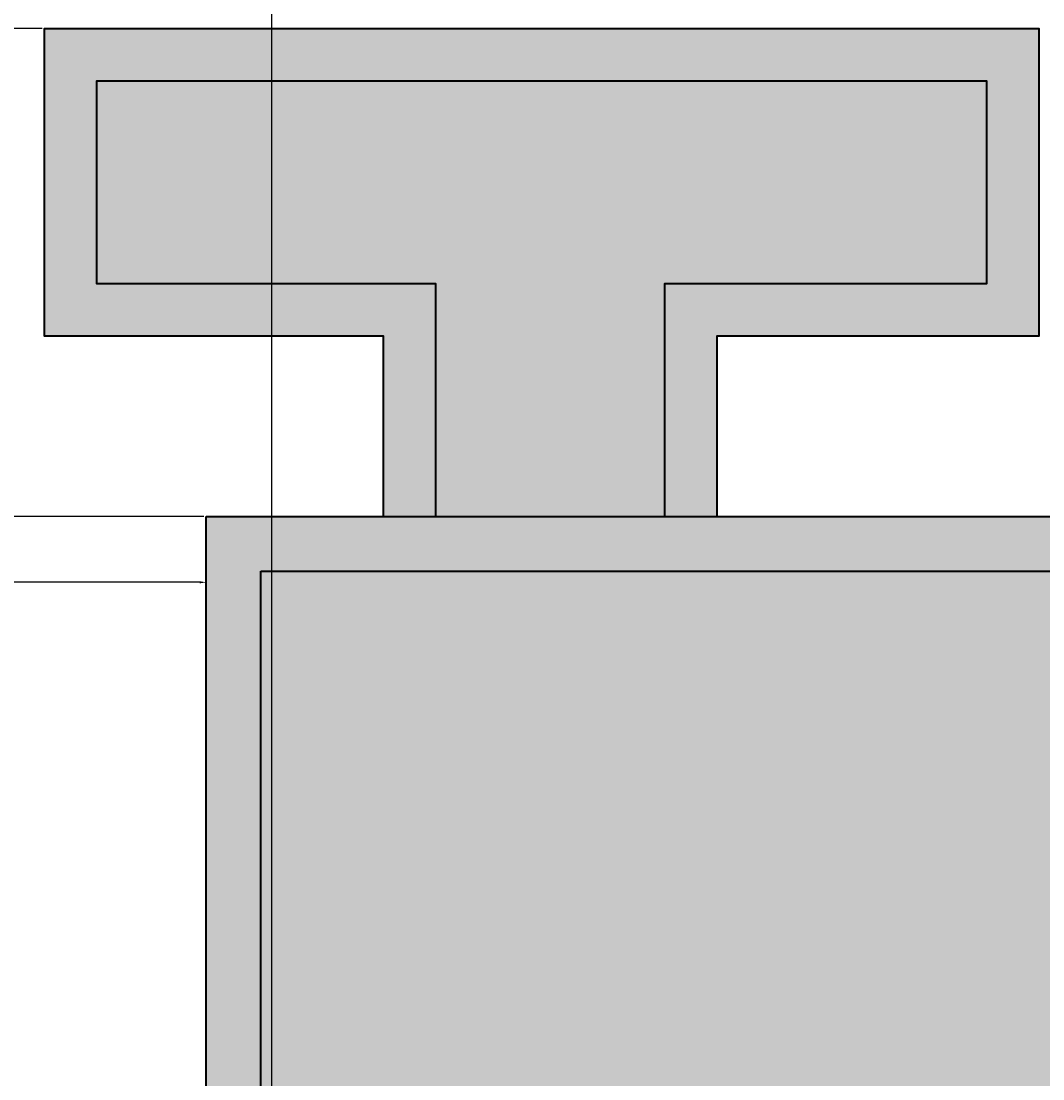
# Model space of a CAD drawing. Units: millimetres. Extents: x -11 to 280, y -4 to 208.
# Tile 15 of 55: x 24 to 52, y 164 to 193. Entities that reach past the tile are written whole.
import ezdxf

# ---------------------------------------------------------------- set-up
doc = ezdxf.new("R2010")
doc.units = ezdxf.units.MM
for name, color, linetype, lineweight in [('M-DIMS', 2, 'Continuous', 18), ('M-HYDR-EQPM', 7, 'Continuous', 35), ('M-HYDR-EQPM-PATT', 252, 'Continuous', 13)]:
    doc.layers.add(name, color=color, linetype=linetype, lineweight=lineweight)
doc.styles.get("Standard").update_dxf_attribs({"font": 'arial.ttf'})
doc.dimstyles.get("Standard").update_dxf_attribs({"dimtxt": 0.18, "dimasz": 0.18, "dimexe": 0.18, "dimexo": 0.0625, "dimgap": 0.09, "dimtad": 0, "dimtih": 1, "dimtoh": 1, "dimdec": 4, "dimzin": 0, "dimdsep": 46, "dimtxsty": 'Standard', "dimcen": 0.09, "dimadec": 0, "dimazin": 0, "dimtfac": 1, "dimtdec": 4, "dimtofl": 0, "dimtmove": 0, "dimatfit": 3, "dimfxl": 1, "dimtolj": 1, "dimtzin": 0, "dimarcsym": 0})

# ---------------------------------------------------------------- blocks, each defined once
blk = doc.blocks.new('*D5')
at = {"layer": 'Defpoints', "color": 0, "transparency": 16777216}
for p in [(24.759, 192.645), (-10.087, 11.435), (261.686, 11.435)]:
    blk.add_point(p, dxfattribs=at)
at = {"layer": 'M-DIMS', "color": 0, "lineweight": -2, "transparency": 16777216}
for p, q in [((24.696, 192.645), (-10.267, 192.645)), ((-10.087, 192.465), (-10.087, 102.222)), ((-10.087, 11.615), (-10.087, 101.858)), ((261.624, 11.435), (-10.267, 11.435))]:
    blk.add_line(p, q, dxfattribs=at)
at = {"layer": 'M-DIMS', "color": 0, "transparency": 16777216}
for points in [[(-10.117, 192.465), (-10.057, 192.465), (-10.087, 192.645)], [(-10.117, 11.615), (-10.057, 11.615), (-10.087, 11.435)]]:
    blk.add_solid(points, dxfattribs=at)
at = {"layer": 'M-DIMS', "color": 0, "transparency": 16777216, "insert": (-10.087, 102.04), "char_height": 0.18, "attachment_point": 5}
blk.add_mtext('\\A1;181.2', dxfattribs=at)
blk = doc.blocks.new('*D8')
at = {"layer": 'Defpoints', "color": 0, "transparency": 16777216}
for p in [(29.201, 177.431), (14.47, 162.581), (29.201, 162.581)]:
    blk.add_point(p, dxfattribs=at)
at = {"layer": 'M-DIMS', "color": 0, "lineweight": -2, "transparency": 16777216}
for p, q in [((14.47, 162.644), (14.47, 177.611)), ((29.201, 162.644), (29.201, 177.611)), ((14.65, 177.431), (21.451, 177.431)), ((29.021, 177.431), (22.221, 177.431))]:
    blk.add_line(p, q, dxfattribs=at)
at = {"layer": 'M-DIMS', "color": 0, "transparency": 16777216}
for points in [[(14.65, 177.461), (14.65, 177.401), (14.47, 177.431)], [(29.021, 177.461), (29.021, 177.401), (29.201, 177.431)]]:
    blk.add_solid(points, dxfattribs=at)
at = {"layer": 'M-DIMS', "color": 0, "transparency": 16777216, "insert": (21.836, 177.431), "char_height": 0.18, "attachment_point": 5}
blk.add_mtext('\\A1;14.73', dxfattribs=at)
blk = doc.blocks.new('*D9')
at = {"layer": 'Defpoints', "color": 0, "transparency": 16777216}
for p in [(78.827, 207.495), (31.006, 98.021), (78.827, 98.149)]:
    blk.add_point(p, dxfattribs=at)
at = {"layer": 'M-DIMS', "color": 0, "lineweight": -2, "transparency": 16777216}
for p, q in [((31.006, 98.084), (31.006, 207.675)), ((31.186, 207.495), (54.52, 207.495)), ((78.647, 207.495), (55.313, 207.495)), ((78.827, 98.212), (78.827, 207.675))]:
    blk.add_line(p, q, dxfattribs=at)
at = {"layer": 'M-DIMS', "color": 0, "transparency": 16777216}
for points in [[(31.186, 207.525), (31.186, 207.465), (31.006, 207.495)], [(78.647, 207.525), (78.647, 207.465), (78.827, 207.495)]]:
    blk.add_solid(points, dxfattribs=at)
at = {"layer": 'M-DIMS', "color": 0, "transparency": 16777216, "insert": (54.917, 207.495), "char_height": 0.18, "attachment_point": 5}
blk.add_mtext('\\A1;47.82', dxfattribs=at)
blk = doc.blocks.new('*D24')
at = {"layer": 'Defpoints', "color": 0, "transparency": 16777216}
for p in [(14.351, 179.241), (29.201, 179.241), (29.201, 153.977)]:
    blk.add_point(p, dxfattribs=at)
at = {"layer": 'M-DIMS', "color": 0, "lineweight": -2, "transparency": 16777216}
for p, q in [((29.139, 179.241), (14.171, 179.241)), ((14.351, 179.061), (14.351, 166.791)), ((14.351, 154.157), (14.351, 166.427)), ((29.139, 153.977), (14.171, 153.977))]:
    blk.add_line(p, q, dxfattribs=at)
at = {"layer": 'M-DIMS', "color": 0, "transparency": 16777216}
for points in [[(14.321, 179.061), (14.381, 179.061), (14.351, 179.241)], [(14.321, 154.157), (14.381, 154.157), (14.351, 153.977)]]:
    blk.add_solid(points, dxfattribs=at)
at = {"layer": 'M-DIMS', "color": 0, "transparency": 16777216, "insert": (14.351, 166.609), "char_height": 0.18, "attachment_point": 5}
blk.add_mtext('\\A1;25.264', dxfattribs=at)

msp = doc.modelspace()

# ---------------------------------------------------------------- hatches: boundary and pattern name
at = {"layer": 'M-HYDR-EQPM-PATT'}
h = msp.add_hatch(color=256, dxfattribs=at)
h.set_gradient(color1=(153, 153, 0), color2=(255, 255, 0), tint=1, name='INVCYLINDER')
h.paths.add_polyline_path([(64.8875, 177.7412), (30.7015, 177.7412), (30.7015, 155.4768), (64.8875, 155.4768)])
h.paths.add_polyline_path([(52.0736, 184.1929), (52.0736, 192.645), (24.7588, 192.645), (24.7588, 184.1929), (34.0713, 184.1929), (34.0713, 179.2412), (35.5061, 179.2412), (35.5061, 185.6276), (26.1935, 185.6276), (26.1935, 191.2103), (50.6389, 191.2103), (50.6389, 185.6276), (41.792, 185.6276), (41.792, 179.2412), (43.2268, 179.2412), (43.2268, 184.1929)])
h = msp.add_hatch(color=256, dxfattribs=at)
h.set_gradient(color1=(153, 153, 0), color2=(153, 153, 0), tint=1, name='INVCYLINDER')
h.paths.add_polyline_path([(26.1935, 191.2103), (26.1935, 185.6276), (35.5061, 185.6276), (35.5061, 179.2412), (41.792, 179.2412), (41.792, 185.6276), (50.6389, 185.6276), (50.6389, 191.2103)])
h.paths.add_polyline_path([(29.2015, 153.9768), (66.3875, 153.9768), (66.3875, 179.2412), (29.2015, 179.2412)])
h.paths.add_polyline_path([(30.7015, 177.7412), (64.8875, 177.7412), (64.8875, 155.4768), (30.7015, 155.4768)], flags=16)

# ---------------------------------------------------------------- linework, layer by layer
at = {"layer": 'M-HYDR-EQPM'}
for points in [[(34.0713, 179.2412), (34.0713, 184.1929), (24.7588, 184.1929), (24.7588, 192.645), (52.0736, 192.645), (52.0736, 184.1929), (43.2268, 184.1929), (43.2268, 179.2412)], [(35.5061, 179.2412), (35.5061, 185.6276), (26.1935, 185.6276), (26.1935, 191.2103), (50.6389, 191.2103), (50.6389, 185.6276), (41.792, 185.6276), (41.792, 179.2412)]]:
    msp.add_lwpolyline(points, dxfattribs=at)
for points in [[(29.2015, 179.2412), (66.3875, 179.2412), (66.3875, 153.9768), (29.2015, 153.9768)], [(30.7015, 177.7412), (64.8875, 177.7412), (64.8875, 155.4768), (30.7015, 155.4768)]]:
    msp.add_lwpolyline(points, close=True, dxfattribs=at)

# ---------------------------------------------------------------- dimensions: what is measured, and where the dimension line sits
at = {"layer": 'M-DIMS'}
for base, p1, p2, picture, middle in [((78.8273, 207.495), (31.0059, 98.0213), (78.8273, 98.1491), '*D9', (54.9166, 207.495)), ((29.2015, 177.4314), (14.4701, 162.5814), (29.2015, 162.5814), '*D8', (21.8358, 177.4314))]:
    dim = msp.add_linear_dim(base=base, p1=p1, p2=p2, dimstyle='Standard', override={"dimdec": 2, "dimlfac": 1, "dimrnd": 0, "dimzin": 0, "dimdsep": 46, "dimlunit": 2}, dxfattribs=at)
    dim.commit()
    dim.dimension.update_dxf_attribs({"geometry": picture, "text_midpoint": middle})
for base, p1, p2, override, picture, middle in [((-10.0865, 11.4346), (24.7588, 192.645), (261.6863, 11.4346), {"dimdec": 1, "dimlfac": 1, "dimrnd": 0, "dimzin": 0, "dimdsep": 46, "dimlunit": 2}, '*D5', (-10.0865, 102.0398)), ((14.3515, 179.2412), (29.2015, 153.9768), (29.2015, 179.2412), {"dimdec": 3, "dimlfac": 1, "dimrnd": 0, "dimzin": 0, "dimdsep": 46, "dimlunit": 2}, '*D24', (14.3515, 166.609))]:
    dim = msp.add_linear_dim(base=base, p1=p1, p2=p2, angle=90, dimstyle='Standard', override=override, dxfattribs=at)
    dim.commit()
    dim.dimension.update_dxf_attribs({"geometry": picture, "text_midpoint": middle})

doc.saveas('drawing.dxf')
